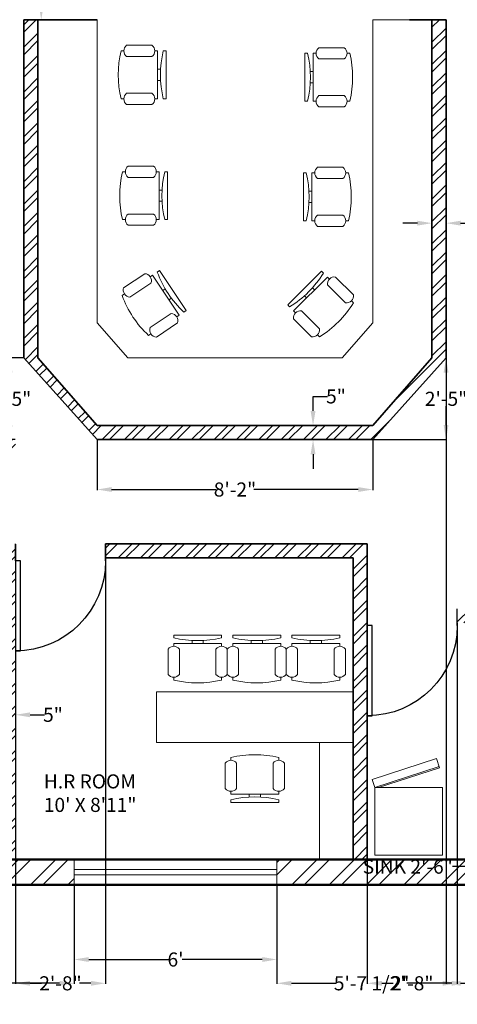
# Model space of a CAD drawing. Units: inches. Extents: x -355 to 263, y -871 to -163.
# Tile 2 of 6: x -133 to 23, y -871 to -521. Entities that reach past the tile are written whole.
import ezdxf

# ---------------------------------------------------------------- set-up
doc = ezdxf.new("R2010")
doc.units = ezdxf.units.IN
doc.header["$MEASUREMENT"] = 0
doc.layers.get('Defpoints').update_dxf_attribs({"color": 50})
for name, color, linetype, lineweight in [('A-ANNO-DIMS', 2, 'Continuous', 18), ('A-AREA-IDEN', 7, 'Continuous', 18), ('A-EQPM', 8, 'Continuous', 18), ('A-WALL-PATT', 252, 'Continuous', 13)]:
    doc.layers.add(name, color=color, linetype=linetype, lineweight=lineweight)
for name, color, linetype, lineweight, plot in [('CHAIR', 8, 'Continuous', 18, False), ('DOOR', 4, 'Continuous', 25, False), ('IWAL', 7, 'Continuous', 35, False), ('OWALL', 7, 'Continuous', 50, False), ('TABLE', 8, 'Continuous', 18, False), ('WIND', 3, 'Continuous', 18, False)]:
    doc.layers.add(name, color=color, linetype=linetype, lineweight=lineweight, plot=plot)
doc.styles.get("Standard").update_dxf_attribs({"font": 'arial.ttf'})
doc.dimstyles.get("Standard").update_dxf_attribs({"dimtxt": 5, "dimasz": 5.18, "dimexe": 0.18, "dimexo": 0.0625, "dimgap": 0.09, "dimtad": 0, "dimtih": 1, "dimtoh": 1, "dimdec": 0, "dimzin": 0, "dimdsep": 46, "dimlunit": 3, "dimtxsty": 'Standard', "dimcen": 0.09, "dimadec": 0, "dimazin": 0, "dimtfac": 1, "dimtdec": 0, "dimtofl": 0, "dimtmove": 0, "dimatfit": 3, "dimfxl": 1, "dimtolj": 1, "dimtzin": 0, "dimarcsym": 0})

# ---------------------------------------------------------------- blocks, each defined once
blk = doc.blocks.new('*U6')
for p, q in [((0, 0), (0, -6)), ((32, 0), (32, -6))]:
    blk.add_line(p, q)
blk.add_lwpolyline([(0, 0), (0, 32), (1.75, 32), (1.75, 0)], close=True)
blk.add_arc((0, 0), 32, 0, 90)
blk = doc.blocks.new('Chair - Desk')
for p, q in [((-8.5, 0), (-8.5, -1)), ((-8.5, 0), (8.5, 0)), ((8.5, 0), (8.5, -1)), ((-8.5, -3), (-8.5, -4)), ((-8.5, -3), (8.5, -3)), ((-2, -3), (-2, -1.9355)), ((2, -1.9576), (2, -3)), ((8.5, -3), (8.5, -4)), ((-10.5, -5), (-10.5, -14)), ((-6.5, -14), (-6.5, -5)), ((6.5, -5), (6.5, -14)), ((10.5, -14), (10.5, -5)), ((-8.5, -15), (-8.5, -16)), ((8.5, -15), (8.5, -16))]:
    blk.add_line(p, q)
for centre, radius, start, end in [((0, 34.625), 36.625, 256.5803, 283.4197), ((-8.5, -6.5), 2.5, 36.8699, 143.1301), ((8.5, -6.5), 2.5, 36.8699, 143.1301), ((-8.5, -12.5), 2.5, 216.8699, 323.1301), ((0, 19.625), 36.625, 256.5803, 283.4197), ((8.5, -12.5), 2.5, 216.8699, 323.1301)]:
    blk.add_arc(centre, radius, start, end)
blk = doc.blocks.new('*D12')
at = {"layer": 'A-ANNO-DIMS', "color": 0, "lineweight": -2, "transparency": 16777216}
for p, q in [((-113.45, -828.34), (-113.45, -854.96)), ((-41.45, -828.34), (-41.45, -854.96)), ((-108.27, -854.78), (-79.86, -854.78)), ((-46.63, -854.78), (-75.05, -854.78))]:
    blk.add_line(p, q, dxfattribs=at)
at = {"layer": 'A-ANNO-DIMS', "color": 0, "lineweight": -3, "transparency": 16777216}
for points in [[(-108.27, -853.92), (-108.27, -855.65), (-113.45, -854.78)], [(-46.63, -853.92), (-46.63, -855.65), (-41.45, -854.78)]]:
    blk.add_solid(points, dxfattribs=at)
at = {"layer": 'Defpoints', "color": 0, "lineweight": -3, "transparency": 16777216}
for p in [(-113.45, -828.28), (-41.45, -828.28), (-41.45, -854.78)]:
    blk.add_point(p, dxfattribs=at)
at = {"layer": 'A-ANNO-DIMS', "color": 0, "transparency": 16777216, "insert": (-77.45, -854.78), "char_height": 5, "attachment_point": 5}
blk.add_mtext("\\A1;6'", dxfattribs=at)
blk = doc.blocks.new('*D48')
at = {"layer": 'A-ANNO-DIMS', "color": 0, "lineweight": -2, "transparency": 16777216}
for p, q in [((-139.32, -763.34), (-139.32, -768.11)), ((-134.32, -763.34), (-134.32, -768.11)), ((-144.5, -767.93), (-149.68, -767.93)), ((-129.14, -767.93), (-123.96, -767.93))]:
    blk.add_line(p, q, dxfattribs=at)
at = {"layer": 'A-ANNO-DIMS', "color": 0, "lineweight": -3, "transparency": 16777216}
for points in [[(-144.5, -767.07), (-144.5, -768.79), (-139.32, -767.93)], [(-129.14, -767.07), (-129.14, -768.79), (-134.32, -767.93)]]:
    blk.add_solid(points, dxfattribs=at)
at = {"layer": 'Defpoints', "color": 0, "lineweight": -3, "transparency": 16777216}
for p in [(-139.32, -763.28), (-134.32, -763.28), (-134.32, -767.93)]:
    blk.add_point(p, dxfattribs=at)
at = {"layer": 'A-ANNO-DIMS', "color": 0, "transparency": 16777216, "insert": (-121, -767.93), "char_height": 5, "attachment_point": 5}
blk.add_mtext('\\A1;5"', dxfattribs=at)
blk = doc.blocks.new('*D51')
at = {"layer": 'A-ANNO-DIMS', "color": 0, "lineweight": -2, "transparency": 16777216}
for p, q in [((-126.26, -485.28), (-124.98, -485.28)), ((-125.16, -490.46), (-125.16, -500.64)), ((-125.16, -516.1), (-125.16, -505.92)), ((-126.26, -521.28), (-124.98, -521.28))]:
    blk.add_line(p, q, dxfattribs=at)
at = {"layer": 'A-ANNO-DIMS', "color": 0, "lineweight": -3, "transparency": 16777216}
for points in [[(-126.02, -490.46), (-124.3, -490.46), (-125.16, -485.28)], [(-126.02, -516.1), (-124.3, -516.1), (-125.16, -521.28)]]:
    blk.add_solid(points, dxfattribs=at)
at = {"layer": 'Defpoints', "color": 0, "lineweight": -3, "transparency": 16777216}
for p in [(-126.32, -485.28), (-125.16, -485.28), (-126.32, -521.28)]:
    blk.add_point(p, dxfattribs=at)
at = {"layer": 'A-ANNO-DIMS', "color": 0, "transparency": 16777216, "insert": (-125.16, -503.28), "char_height": 5, "attachment_point": 5}
blk.add_mtext("\\A1;3'", dxfattribs=at)
blk = doc.blocks.new('*D53')
at = {"layer": 'A-ANNO-DIMS', "color": 0, "lineweight": -2, "transparency": 16777216}
for p, q in [((-131.38, -641.28), (-136.42, -641.28)), ((-136.24, -646.46), (-136.24, -653.14)), ((-136.24, -665.1), (-136.24, -658.42)), ((-134.38, -670.28), (-136.42, -670.28))]:
    blk.add_line(p, q, dxfattribs=at)
at = {"layer": 'A-ANNO-DIMS', "color": 0, "lineweight": -3, "transparency": 16777216}
for points in [[(-137.1, -646.46), (-135.38, -646.46), (-136.24, -641.28)], [(-137.1, -665.1), (-135.38, -665.1), (-136.24, -670.28)]]:
    blk.add_solid(points, dxfattribs=at)
at = {"layer": 'Defpoints', "color": 0, "lineweight": -3, "transparency": 16777216}
for p in [(-136.24, -641.28), (-131.32, -641.28), (-134.32, -670.28)]:
    blk.add_point(p, dxfattribs=at)
at = {"layer": 'A-ANNO-DIMS', "color": 0, "transparency": 16777216, "insert": (-136.24, -655.78), "char_height": 5, "attachment_point": 5}
blk.add_mtext('\\A1;2\'-5"', dxfattribs=at)
blk = doc.blocks.new('*D54')
at = {"layer": 'A-ANNO-DIMS', "color": 0, "lineweight": -2, "transparency": 16777216}
for p, q in [((-105.32, -670.34), (-105.32, -688.16)), ((-7.32, -670.34), (-7.32, -688.16)), ((-100.14, -687.98), (-63.06, -687.98)), ((-12.5, -687.98), (-49.58, -687.98))]:
    blk.add_line(p, q, dxfattribs=at)
at = {"layer": 'A-ANNO-DIMS', "color": 0, "lineweight": -3, "transparency": 16777216}
for points in [[(-100.14, -687.11), (-100.14, -688.84), (-105.32, -687.98)], [(-12.5, -687.11), (-12.5, -688.84), (-7.32, -687.98)]]:
    blk.add_solid(points, dxfattribs=at)
at = {"layer": 'Defpoints', "color": 0, "lineweight": -3, "transparency": 16777216}
for p in [(-105.32, -670.28), (-7.32, -670.28), (-7.32, -687.98)]:
    blk.add_point(p, dxfattribs=at)
at = {"layer": 'A-ANNO-DIMS', "color": 0, "transparency": 16777216, "insert": (-56.32, -687.98), "char_height": 5, "attachment_point": 5}
blk.add_mtext('\\A1;8\'-2"', dxfattribs=at)
blk = doc.blocks.new('*D55')
at = {"layer": 'A-ANNO-DIMS', "color": 0, "lineweight": -2, "transparency": 16777216}
for p, q in [((18.62, -641.28), (18.5, -641.28)), ((18.68, -646.46), (18.68, -653.14)), ((18.68, -665.1), (18.68, -658.42)), ((-7.26, -670.28), (18.86, -670.28))]:
    blk.add_line(p, q, dxfattribs=at)
at = {"layer": 'A-ANNO-DIMS', "color": 0, "lineweight": -3, "transparency": 16777216}
for points in [[(17.82, -646.46), (19.54, -646.46), (18.68, -641.28)], [(17.82, -665.1), (19.54, -665.1), (18.68, -670.28)]]:
    blk.add_solid(points, dxfattribs=at)
at = {"layer": 'Defpoints', "color": 0, "lineweight": -3, "transparency": 16777216}
for p in [(18.68, -641.28), (18.68, -641.28), (-7.32, -670.28)]:
    blk.add_point(p, dxfattribs=at)
at = {"layer": 'A-ANNO-DIMS', "color": 0, "transparency": 16777216, "insert": (18.68, -655.78), "char_height": 5, "attachment_point": 5}
blk.add_mtext('\\A1;2\'-5"', dxfattribs=at)
blk = doc.blocks.new('*D56')
at = {"layer": 'A-ANNO-DIMS', "color": 0, "lineweight": -2, "transparency": 16777216}
for p, q in [((8.5, -593.44), (3.32, -593.44)), ((13.68, -595.07), (13.68, -593.26)), ((18.68, -595.07), (18.68, -593.26)), ((23.86, -593.44), (29.04, -593.44))]:
    blk.add_line(p, q, dxfattribs=at)
at = {"layer": 'A-ANNO-DIMS', "color": 0, "lineweight": -3, "transparency": 16777216}
for points in [[(8.5, -592.58), (8.5, -594.3), (13.68, -593.44)], [(23.86, -592.58), (23.86, -594.3), (18.68, -593.44)]]:
    blk.add_solid(points, dxfattribs=at)
at = {"layer": 'Defpoints', "color": 0, "lineweight": -3, "transparency": 16777216}
for p in [(18.68, -593.44), (13.68, -595.13), (18.68, -595.13)]:
    blk.add_point(p, dxfattribs=at)
at = {"layer": 'A-ANNO-DIMS', "color": 0, "transparency": 16777216, "insert": (32, -593.44), "char_height": 5, "attachment_point": 5}
blk.add_mtext('\\A1;5"', dxfattribs=at)
blk = doc.blocks.new('*D57')
at = {"layer": 'A-ANNO-DIMS', "color": 0, "lineweight": -2, "transparency": 16777216}
for p, q in [((-28.58, -660.1), (-28.58, -654.92)), ((-28.58, -654.92), (-23.4, -654.92)), ((-28.77, -665.28), (-28.4, -665.28)), ((-28.77, -670.28), (-28.4, -670.28)), ((-28.58, -675.46), (-28.58, -680.64))]:
    blk.add_line(p, q, dxfattribs=at)
at = {"layer": 'A-ANNO-DIMS', "color": 0, "lineweight": -3, "transparency": 16777216}
for points in [[(-29.45, -660.1), (-27.72, -660.1), (-28.58, -665.28)], [(-29.45, -675.46), (-27.72, -675.46), (-28.58, -670.28)]]:
    blk.add_solid(points, dxfattribs=at)
at = {"layer": 'Defpoints', "color": 0, "lineweight": -3, "transparency": 16777216}
for p in [(-28.83, -665.28), (-28.58, -665.28), (-28.83, -670.28)]:
    blk.add_point(p, dxfattribs=at)
at = {"layer": 'A-ANNO-DIMS', "color": 0, "transparency": 16777216, "insert": (-20.44, -654.92), "char_height": 5, "attachment_point": 5}
blk.add_mtext('\\A1;5"', dxfattribs=at)
blk = doc.blocks.new('*D71')
at = {"layer": 'A-ANNO-DIMS', "color": 0, "lineweight": -2, "transparency": 16777216}
for p, q in [((26.1, -817.38), (26.1, -822)), ((56.1, -817.38), (56.1, -822)), ((26.1, -821.82), (20.92, -821.82)), ((50.92, -821.82), (31.28, -821.82))]:
    blk.add_line(p, q, dxfattribs=at)
at = {"layer": 'A-ANNO-DIMS', "color": 0, "lineweight": -3, "transparency": 16777216}
for points in [[(31.28, -820.96), (31.28, -822.68), (26.1, -821.82)], [(50.92, -820.96), (50.92, -822.68), (56.1, -821.82)]]:
    blk.add_solid(points, dxfattribs=at)
at = {"layer": 'Defpoints', "color": 0, "lineweight": -3, "transparency": 16777216}
for p in [(26.1, -817.32), (56.1, -817.32), (26.1, -821.82)]:
    blk.add_point(p, dxfattribs=at)
at = {"layer": 'A-ANNO-DIMS', "color": 0, "transparency": 16777216, "insert": (5.07, -821.82), "char_height": 5, "attachment_point": 5}
blk.add_mtext('\\A1;SINK 2\'-6"', dxfattribs=at)
blk = doc.blocks.new('*D82')
at = {"layer": 'A-ANNO-DIMS', "color": 0, "lineweight": -2, "transparency": 16777216}
for p, q in [((-301.32, -828.34), (-301.32, -863.41)), ((-113.45, -828.34), (-113.45, -863.41)), ((-296.14, -863.23), (-215.83, -863.23)), ((-118.63, -863.23), (-198.94, -863.23))]:
    blk.add_line(p, q, dxfattribs=at)
at = {"layer": 'A-ANNO-DIMS', "color": 0, "lineweight": -3, "transparency": 16777216}
for points in [[(-296.14, -862.37), (-296.14, -864.09), (-301.32, -863.23)], [(-118.63, -862.37), (-118.63, -864.09), (-113.45, -863.23)]]:
    blk.add_solid(points, dxfattribs=at)
at = {"layer": 'Defpoints', "color": 0, "lineweight": -3, "transparency": 16777216}
for p in [(-301.32, -828.28), (-113.45, -828.28), (-113.45, -863.23)]:
    blk.add_point(p, dxfattribs=at)
at = {"layer": 'A-ANNO-DIMS', "color": 0, "transparency": 16777216, "insert": (-207.39, -863.23), "char_height": 5, "attachment_point": 5}
blk.add_mtext('\\A1;15\'-8"', dxfattribs=at)
blk = doc.blocks.new('*D83')
at = {"layer": 'A-ANNO-DIMS', "color": 0, "lineweight": -2, "transparency": 16777216}
for p, q in [((-41.45, -828.34), (-41.45, -863.41)), ((25.9, -828.34), (25.9, -863.41)), ((-36.27, -863.23), (-20.33, -863.23)), ((20.72, -863.23), (4.79, -863.23))]:
    blk.add_line(p, q, dxfattribs=at)
at = {"layer": 'A-ANNO-DIMS', "color": 0, "lineweight": -3, "transparency": 16777216}
for points in [[(-36.27, -862.37), (-36.27, -864.09), (-41.45, -863.23)], [(20.72, -862.37), (20.72, -864.09), (25.9, -863.23)]]:
    blk.add_solid(points, dxfattribs=at)
at = {"layer": 'Defpoints', "color": 0, "lineweight": -3, "transparency": 16777216}
for p in [(-41.45, -828.28), (25.9, -828.28), (25.9, -863.23)]:
    blk.add_point(p, dxfattribs=at)
at = {"layer": 'A-ANNO-DIMS', "color": 0, "transparency": 16777216, "insert": (-7.77, -863.23), "char_height": 5, "attachment_point": 5}
blk.add_mtext('\\A1;5\'-7 1/2"', dxfattribs=at)
blk = doc.blocks.new('*D86')
at = {"layer": 'A-ANNO-DIMS', "color": 0, "lineweight": -2, "transparency": 16777216}
for p, q in [((18.68, -641.34), (18.68, -863.41)), ((54.68, -665.34), (54.68, -863.41)), ((23.86, -863.23), (29.95, -863.23)), ((49.5, -863.23), (43.41, -863.23))]:
    blk.add_line(p, q, dxfattribs=at)
at = {"layer": 'A-ANNO-DIMS', "color": 0, "lineweight": -3, "transparency": 16777216}
for points in [[(23.86, -862.37), (23.86, -864.09), (18.68, -863.23)], [(49.5, -862.37), (49.5, -864.09), (54.68, -863.23)]]:
    blk.add_solid(points, dxfattribs=at)
at = {"layer": 'Defpoints', "color": 0, "lineweight": -3, "transparency": 16777216}
for p in [(18.68, -641.28), (54.68, -665.28), (54.68, -863.23)]:
    blk.add_point(p, dxfattribs=at)
at = {"layer": 'A-ANNO-DIMS', "color": 0, "transparency": 16777216, "insert": (36.68, -863.23), "char_height": 5, "attachment_point": 5}
blk.add_mtext('\\A1;3\'-0"', dxfattribs=at)
blk = doc.blocks.new('*D88')
at = {"layer": 'A-ANNO-DIMS', "color": 0, "lineweight": -2, "transparency": 16777216}
for p, q in [((-134.32, -707.34), (-134.32, -863.41)), ((-102.32, -707.34), (-102.32, -863.41)), ((-129.14, -863.23), (-125.1, -863.23)), ((-107.5, -863.23), (-111.54, -863.23))]:
    blk.add_line(p, q, dxfattribs=at)
at = {"layer": 'A-ANNO-DIMS', "color": 0, "lineweight": -3, "transparency": 16777216}
for points in [[(-129.14, -862.37), (-129.14, -864.09), (-134.32, -863.23)], [(-107.5, -862.37), (-107.5, -864.09), (-102.32, -863.23)]]:
    blk.add_solid(points, dxfattribs=at)
at = {"layer": 'Defpoints', "color": 0, "lineweight": -3, "transparency": 16777216}
for p in [(-134.32, -707.28), (-102.32, -707.28), (-102.32, -863.23)]:
    blk.add_point(p, dxfattribs=at)
at = {"layer": 'A-ANNO-DIMS', "color": 0, "transparency": 16777216, "insert": (-118.32, -863.23), "char_height": 5, "attachment_point": 5}
blk.add_mtext('\\A1;2\'-8"', dxfattribs=at)
blk = doc.blocks.new('*D89')
at = {"layer": 'A-ANNO-DIMS', "color": 0, "lineweight": -2, "transparency": 16777216}
for p, q in [((-9.32, -736.34), (-9.32, -863.41)), ((22.68, -735.34), (22.68, -863.41)), ((-4.14, -863.23), (-0.1, -863.23)), ((17.5, -863.23), (13.46, -863.23))]:
    blk.add_line(p, q, dxfattribs=at)
at = {"layer": 'A-ANNO-DIMS', "color": 0, "lineweight": -3, "transparency": 16777216}
for points in [[(-4.14, -862.37), (-4.14, -864.09), (-9.32, -863.23)], [(17.5, -862.37), (17.5, -864.09), (22.68, -863.23)]]:
    blk.add_solid(points, dxfattribs=at)
at = {"layer": 'Defpoints', "color": 0, "lineweight": -3, "transparency": 16777216}
for p in [(-9.32, -736.28), (22.68, -735.28), (22.68, -863.23)]:
    blk.add_point(p, dxfattribs=at)
at = {"layer": 'A-ANNO-DIMS', "color": 0, "transparency": 16777216, "insert": (6.68, -863.23), "char_height": 5, "attachment_point": 5}
blk.add_mtext('\\A1;2\'-8"', dxfattribs=at)

msp = doc.modelspace()

# ---------------------------------------------------------------- hatches: boundary and pattern name
at = {"layer": 'A-WALL-PATT'}
h = msp.add_hatch(dxfattribs=at)
h.set_pattern_fill('ANSI32', color=256, scale=25)
h.set_pattern_definition([(45, (-301.32, -828.28), (-6.62913, 6.62913), []), (45, (-296.9, -828.28), (-6.62913, 6.62913), [])])
h.paths.add_polyline_path([(54.68, -289.28), (-301.32, -289.28), (-301.32, -303.28), (-295.02, -303.28), (-292.32, -303.28), (-292.32, -298.28), (54.68, -298.28)])
h.paths.add_polyline_path([(188.68, -216.28), (54.68, -216.28), (54.68, -225.28), (179.68, -225.28), (179.68, -345.28), (179.68, -485.16), (184.18, -485.16), (188.68, -485.16)])
h.paths.add_polyline_path([(188.68, -521.16), (184.18, -521.16), (179.68, -521.16), (179.68, -540.28), (188.68, -540.28)])
h.paths.add_polyline_path([(164.68, -540.28), (155.68, -540.28), (155.68, -552.97), (160.18, -552.97), (164.68, -552.97)])
h.paths.add_polyline_path([(164.68, -588.97), (160.18, -588.97), (155.68, -588.97), (155.68, -620.04), (160.18, -620.04), (164.68, -620.04)])
h.paths.add_polyline_path([(164.68, -656.04), (160.18, -656.04), (155.68, -656.04), (155.68, -682.06), (160.18, -682.06), (164.68, -682.06)])
h.paths.add_polyline_path([(164.68, -718.06), (160.18, -718.06), (155.68, -718.06), (155.68, -730.28), (164.68, -730.28)])
h.paths.add_polyline_path([(188.68, -730.28), (179.68, -730.28), (179.68, -819.28), (73.9, -819.28), (73.9, -823.78), (73.9, -828.28), (188.68, -828.28)])
h.paths.add_polyline_path([(25.9, -819.28), (-41.45, -819.28), (-41.45, -823.78), (-41.45, -828.28), (25.9, -828.28), (25.9, -823.78)])
h.paths.add_polyline_path([(-113.45, -819.28), (-292.32, -819.28), (-292.32, -796.14), (-296.82, -796.14), (-301.32, -796.14), (-301.32, -828.28), (-113.45, -828.28), (-113.45, -823.78)])
h.paths.add_polyline_path([(-292.32, -480.28), (-292.32, -345.28), (-301.32, -345.28), (-301.32, -620.18), (-296.82, -620.18), (-292.32, -620.18)])
h.paths.add_polyline_path([(-292.32, -656.18), (-296.82, -656.18), (-301.32, -656.18), (-301.32, -700.14), (-296.82, -700.14), (-292.32, -700.14)])
h = msp.add_hatch(dxfattribs=at)
h.set_pattern_fill('ANSI32', color=256, scale=15)
h.set_pattern_definition([(45, (-292.3197, -819.28), (-3.977476, 3.977476), []), (45, (-289.668, -819.28), (-3.977476, 3.977476), [])])
h.paths.add_polyline_path([(59.68, -280.18), (57.18, -280.18), (54.68, -280.18), (54.68, -289.28), (54.68, -298.28), (54.68, -303.28), (59.68, -303.28)])
h.paths.add_polyline_path([(59.68, -225.28), (54.68, -225.28), (54.68, -232.18), (57.18, -232.18), (59.68, -232.18)])
h.paths.add_polyline_path([(18.68, -641.28), (18.68, -521.28), (13.68, -521.28), (13.68, -641.28), (-7.32, -665.28), (-105.32, -665.28), (-126.32, -641.28), (-126.32, -521.28), (-131.32, -521.28), (-131.32, -641.28), (-105.32, -670.28), (-7.32, -670.28)])
h.paths.add_polyline_path([(-167.32, -521.28), (-172.32, -521.28), (-172.32, -538.25), (-169.82, -538.25), (-167.32, -538.25)])
h.paths.add_polyline_path([(-134.32, -670.28), (-167.32, -670.28), (-167.32, -610.28), (-167.32, -586.25), (-169.82, -586.25), (-172.32, -586.25), (-172.32, -670.28), (-292.32, -670.28), (-292.32, -675.28), (-139.32, -675.28), (-134.32, -675.28)])
h.paths.add_polyline_path([(-167.32, -345.28), (-172.32, -345.28), (-172.32, -462.28), (-172.32, -480.28), (-292.32, -480.28), (-292.32, -485.28), (-172.32, -485.28), (-167.32, -485.28), (5.68, -485.28), (5.68, -480.28), (-167.32, -480.28)])
h.paths.add_polyline_path([(179.68, -345.28), (30.68, -345.28), (30.68, -365.65), (33.18, -365.65), (35.68, -365.65), (35.68, -350.28), (179.68, -350.28)])
h.paths.add_polyline_path([(-134.32, -707.28), (-139.32, -707.28), (-139.32, -819.28), (-134.32, -819.28)])
h.paths.add_polyline_path([(-9.32, -707.28), (-102.32, -707.28), (-102.32, -712.28), (-14.32, -712.28), (-14.32, -819.28), (-9.32, -819.28)])
h.paths.add_polyline_path([(179.68, -730.28), (22.68, -730.28), (22.68, -735.28), (179.68, -735.28)])
h.paths.add_polyline_path([(179.68, -470.28), (30.68, -470.28), (30.68, -475.28), (54.68, -475.28), (54.68, -505.29), (59.18, -505.29, -0.00418), (59.68, -505.29), (59.68, -475.28), (179.68, -475.28)])
h.paths.add_polyline_path([(35.68, -413.65), (33.18, -413.65), (30.68, -413.65), (30.68, -440.29), (35.18, -440.29, -0.00418), (35.68, -440.29)])
h.paths.add_polyline_path([(179.68, -535.28), (54.68, -535.28), (54.68, -540.28), (54.68, -570.29), (59.18, -570.29, -0.00418), (59.68, -570.29), (59.68, -540.28), (179.68, -540.28)])
h.paths.add_polyline_path([(121.93, -531.51), (160.73, -531.51), (160.73, -512.85), (121.93, -512.85)], flags=9)
h.paths.add_polyline_path([(49.47, -376.48), (111.2, -376.48), (111.2, -357.82), (49.47, -357.82)], flags=9)

# ---------------------------------------------------------------- linework, layer by layer
at = {"layer": 'A-EQPM'}
for p, q in [((-7.55, -790.87), (15.29, -783.49)), ((15.29, -783.49), (16.33, -786.73)), ((-6.63, -793.73), (16.21, -786.34)), ((-5.33, -793.73), (16.33, -786.73)), ((-7.55, -790.87), (-6.63, -793.73))]:
    msp.add_line(p, q, dxfattribs=at)
msp.add_lwpolyline([(-6.63, -817.73), (17.37, -817.73), (17.37, -793.73), (-6.63, -793.73)], close=True, dxfattribs=at)
at = {"layer": 'IWAL'}
for p, q in [((-131.32, -641.28), (-131.32, -521.28)), ((-105.32, -521.28), (-131.32, -521.28)), ((-126.32, -641.28), (-126.32, -521.28)), ((5.68, -521.28), (18.68, -521.28)), ((13.68, -521.28), (13.68, -641.28)), ((18.68, -521.28), (18.68, -641.28)), ((-105.32, -670.28), (-131.32, -641.28)), ((-126.32, -641.28), (-105.32, -665.28)), ((-7.32, -670.28), (18.68, -641.28)), ((13.68, -641.28), (-7.32, -665.28)), ((-7.32, -665.28), (-105.32, -665.28)), ((-7.32, -670.28), (-105.32, -670.28)), ((-9.32, -707.28), (-102.32, -707.28)), ((-9.32, -707.28), (-9.32, -819.28)), ((-14.32, -712.28), (-102.32, -712.28)), ((-14.32, -712.28), (-14.32, -819.28))]:
    msp.add_line(p, q, dxfattribs=at)
at = {"layer": 'OWALL'}
for p, q in [((179.68, -819.28), (-292.32, -819.28)), ((188.68, -828.28), (-301.32, -828.28))]:
    msp.add_line(p, q, dxfattribs=at)
at = {"layer": 'TABLE'}
for p, q in [((-105.32, -628.83), (-105.32, -521.28)), ((5.68, -521.28), (-7.32, -521.28)), ((-7.32, -521.28), (-7.32, -628.83)), ((-105.32, -628.83), (-94.43, -641.28)), ((-7.32, -628.83), (-18.21, -641.28)), ((-18.21, -641.28), (-94.43, -641.28)), ((-14.32, -759.78), (-84.19, -759.78)), ((-84.19, -759.78), (-84.19, -777.78)), ((-84.19, -777.78), (-14.32, -777.78)), ((-26.32, -777.78), (-26.32, -819.28))]:
    msp.add_line(p, q, dxfattribs=at)
at = {"layer": 'WIND'}
for p, q in [((-113.45, -823.78), (-113.45, -819.28)), ((-41.45, -823.78), (-41.45, -819.28)), ((-113.45, -822.88), (-41.45, -822.88)), ((-113.45, -823.78), (-113.45, -828.28)), ((-113.45, -824.68), (-41.45, -824.68)), ((-41.45, -823.78), (-41.45, -828.28))]:
    msp.add_line(p, q, dxfattribs=at)

# ---------------------------------------------------------------- block references
at = {"layer": 'CHAIR'}
for p, rotation in [((-80.81, -540.82), 270), ((-31.51, -541.66), 90), ((-80.27, -583.69), 270), ((-31.98, -584.08), 90), ((-78.4, -617.35), 303.6027999678462), ((-31.59, -616.44), 44.99999999999978)]:
    msp.add_blockref('Chair - Desk', p, dxfattribs=dict(at, rotation=rotation))
at = {"layer": 'CHAIR', "xscale": -1}
for p in [(-69.58, -739.61), (-48.58, -739.61), (-27.58, -739.61)]:
    msp.add_blockref('Chair - Desk', p, dxfattribs=at)
at = {"layer": 'CHAIR', "xscale": -1, "rotation": 180}
msp.add_blockref('Chair - Desk', (-49.26, -799.09), dxfattribs=at)
at = {"layer": 'DOOR', "xscale": -1, "rotation": 180}
for p in [(-134.32, -713.28), (-9.32, -736.28)]:
    msp.add_blockref('*U6', p, dxfattribs=at)

# ---------------------------------------------------------------- texts
at = {"layer": 'A-AREA-IDEN', "insert": (-124.24, -789.07), "char_height": 5, "attachment_point": 1}
msp.add_mtext_dynamic_manual_height_columns('{H.R ROOM\\P10\' X 8\'11"}', width=50.9885, gutter_width=1, heights=[0], dxfattribs=at)

# ---------------------------------------------------------------- dimensions: what is measured, and where the dimension line sits
at = {"layer": 'A-ANNO-DIMS'}
for base, p1, p2, picture, middle in [((-125.16, -485.28), (-126.32, -521.28), (-126.32, -485.28), '*D51', (-125.16, -503.28)), ((-136.24, -641.28), (-134.32, -670.28), (-131.32, -641.28), '*D53', (-136.24, -655.78)), ((18.68, -641.28), (-7.32, -670.28), (18.68, -641.28), '*D55', (18.68, -655.78)), ((-28.58, -665.28), (-28.83, -670.28), (-28.83, -665.28), '*D57', (-20.44, -654.92))]:
    dim = msp.add_linear_dim(base=base, p1=p1, p2=p2, angle=90, dimstyle='Standard', override={"dimclrd": 0, "dimclre": 0, "dimclrt": 0}, dxfattribs=at)
    dim.commit()
    dim.dimension.update_dxf_attribs({"geometry": picture, "text_midpoint": middle})
for base, p1, p2, override, picture, middle in [((18.68, -593.44), (13.68, -595.13), (18.68, -595.13), {"dimclrd": 0, "dimclre": 0, "dimclrt": 0}, '*D56', (32, -593.44)), ((54.68, -863.23), (18.68, -641.28), (54.68, -665.28), {"dimdec": 1, "dimlfac": 1, "dimrnd": 0, "dimzin": 1, "dimdsep": 46, "dimlunit": 4, "dimfrac": 2}, '*D86', (36.68, -863.23)), ((-102.32, -863.23), (-134.32, -707.28), (-102.32, -707.28), {"dimdec": 1, "dimlfac": 1, "dimrnd": 0, "dimzin": 1, "dimdsep": 46, "dimlunit": 4, "dimfrac": 2}, '*D88', (-118.32, -863.23)), ((22.68, -863.23), (-9.32, -736.28), (22.68, -735.28), {"dimdec": 1, "dimlfac": 1, "dimrnd": 0, "dimzin": 1, "dimdsep": 46, "dimlunit": 4, "dimfrac": 2}, '*D89', (6.68, -863.23)), ((-134.32, -767.93), (-139.32, -763.28), (-134.32, -763.28), {"dimclrd": 0, "dimclre": 0, "dimclrt": 0}, '*D48', (-121, -767.93)), ((-113.45, -863.23), (-301.32, -828.28), (-113.45, -828.28), {"dimdec": 1, "dimlfac": 1, "dimrnd": 0, "dimzin": 1, "dimdsep": 46, "dimlunit": 4, "dimfrac": 2}, '*D82', (-207.39, -863.23)), ((-41.45, -854.78), (-113.45, -828.28), (-41.45, -828.28), {"dimclrd": 0, "dimclre": 0, "dimclrt": 0}, '*D12', (-77.45, -854.78)), ((25.9042, -863.23), (-41.4512, -828.28), (25.9042, -828.28), {"dimdec": 1, "dimlfac": 1, "dimrnd": 0, "dimzin": 1, "dimdsep": 46, "dimlunit": 4, "dimfrac": 2}, '*D83', (-7.7735, -863.23))]:
    dim = msp.add_linear_dim(base=base, p1=p1, p2=p2, dimstyle='Standard', override=override, dxfattribs=at)
    dim.commit()
    dim.dimension.update_dxf_attribs({"geometry": picture, "text_midpoint": middle})
dim = msp.add_linear_dim(base=(-7.32, -687.98), p1=(-105.32, -670.28), p2=(-7.32, -670.28), dimstyle='Standard', override={"dimclrd": 0, "dimclre": 0, "dimclrt": 0}, dxfattribs=at)
dim.commit()
dim.dimension.update_dxf_attribs({"geometry": '*D54', "text_midpoint": (-56.32, -687.98), "dimtype": 160})
dim = msp.add_linear_dim(base=(26.1, -821.82), p1=(56.1, -817.32), p2=(26.1, -817.32), angle=180, text='SINK <>', dimstyle='Standard', override={"dimdec": 1, "dimlfac": 1, "dimrnd": 0, "dimzin": 1, "dimdsep": 46, "dimlunit": 4, "dimfrac": 2}, dxfattribs=at)
dim.commit()
dim.dimension.update_dxf_attribs({"geometry": '*D71', "text_midpoint": (5.07, -821.82)})

doc.saveas('drawing.dxf')
